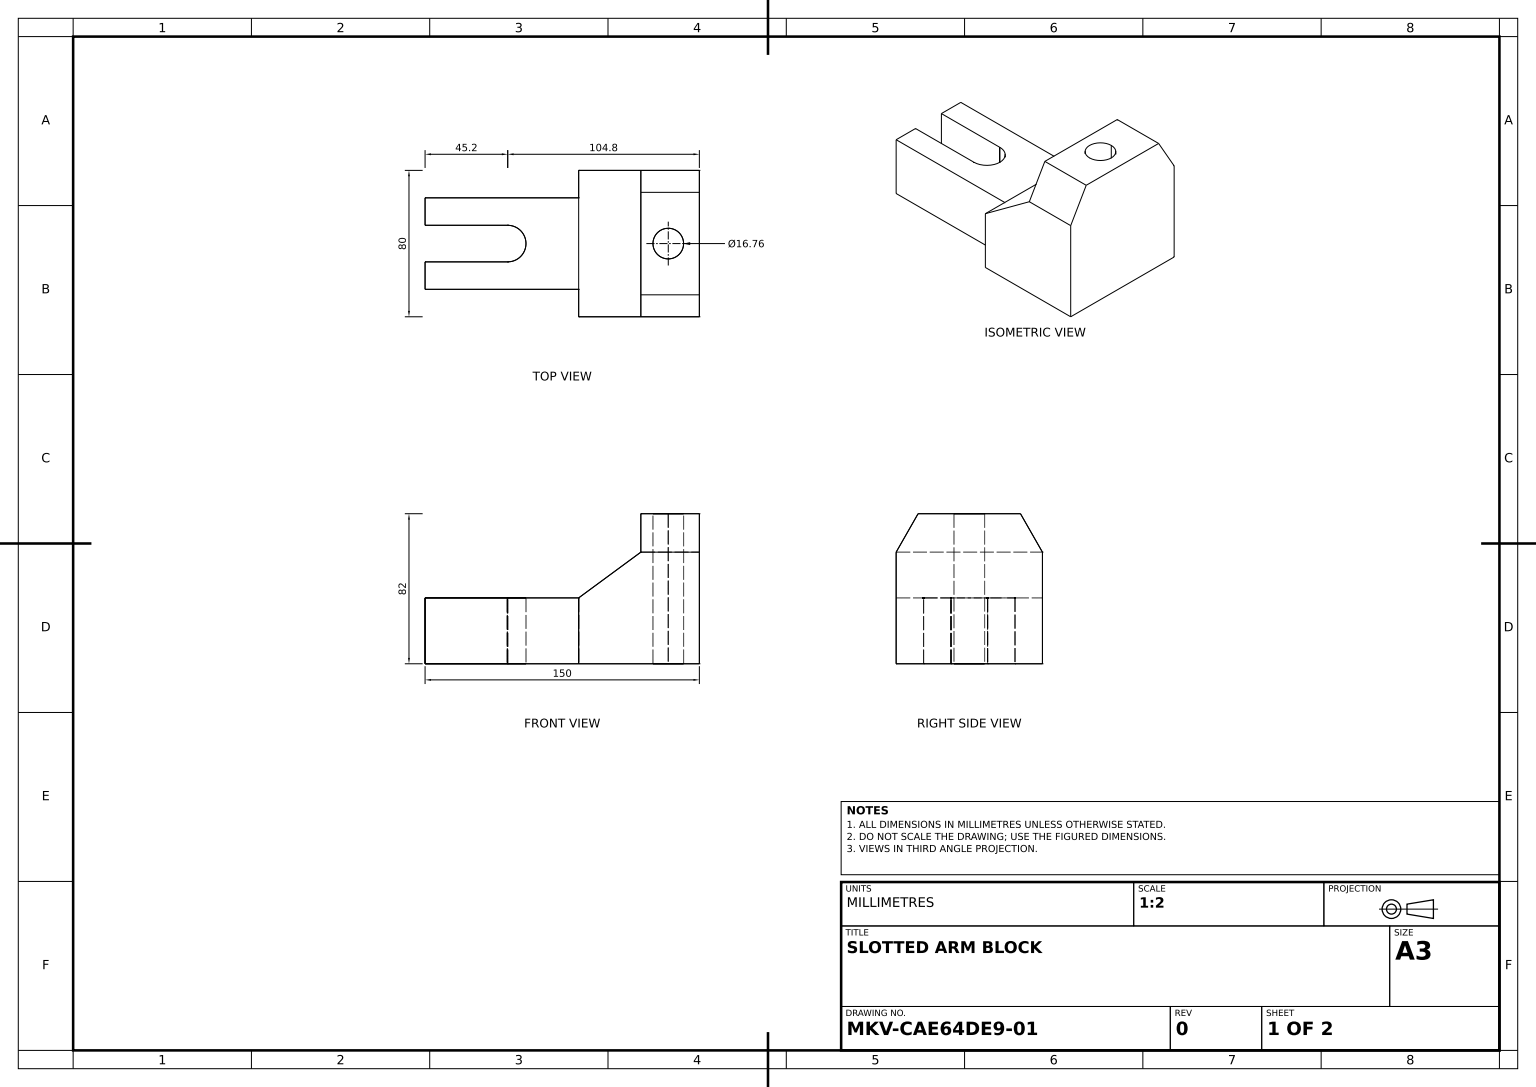
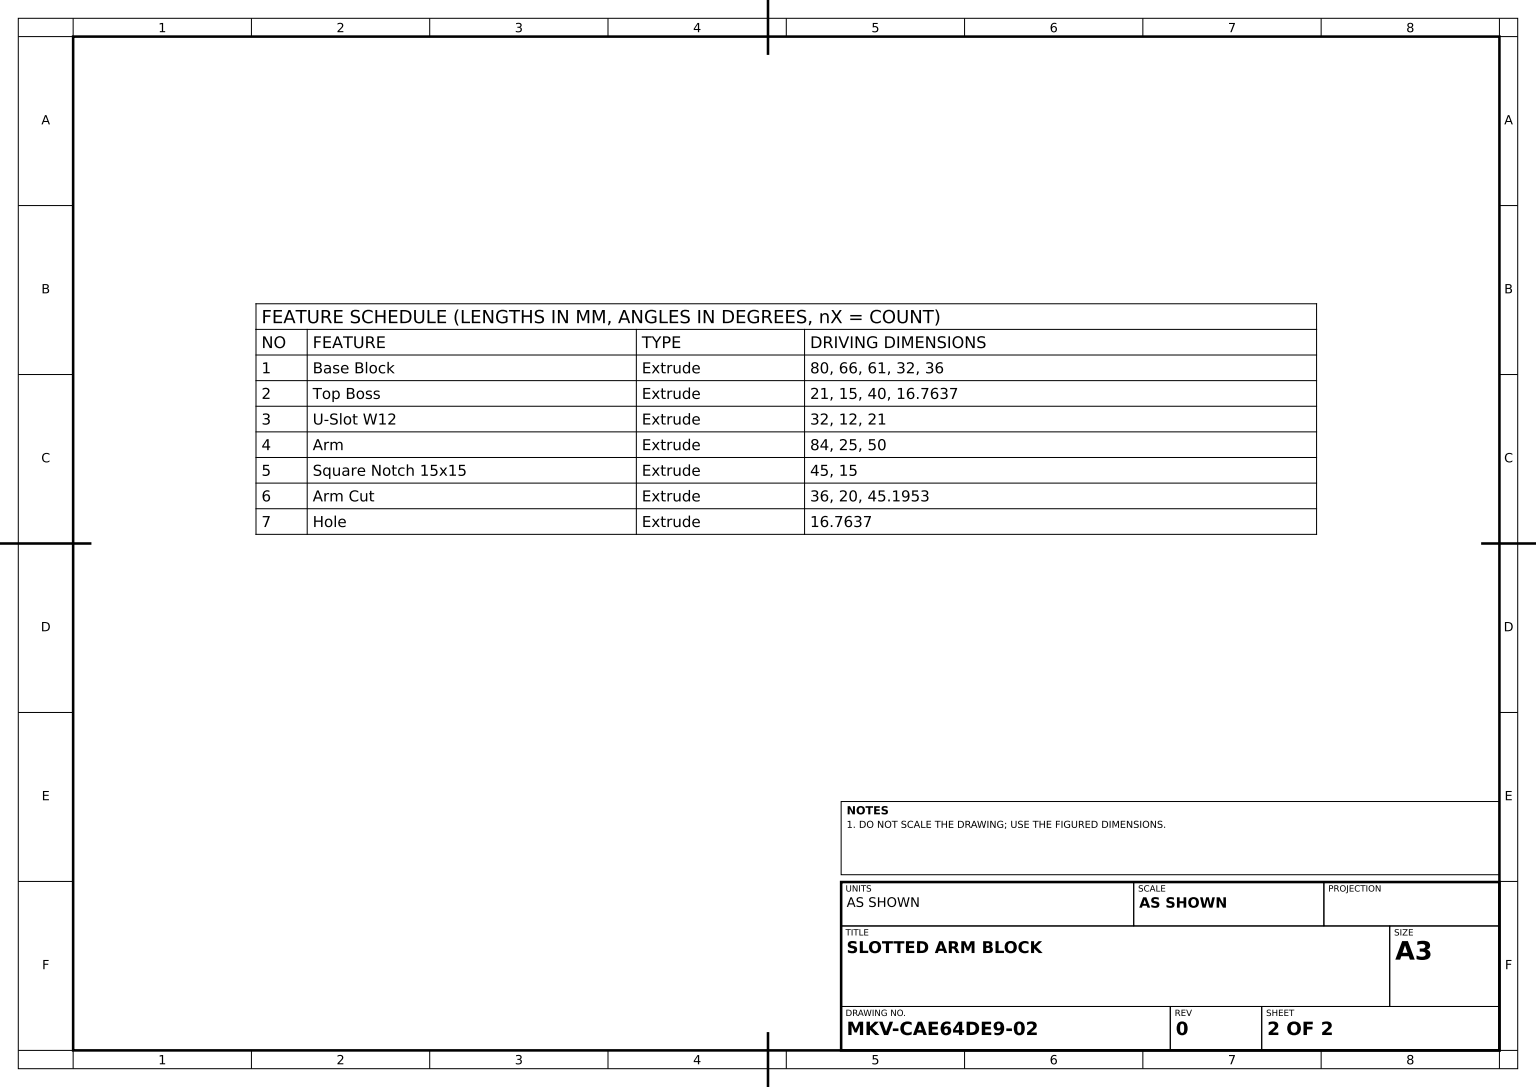
SolidWorks part; units mm, degrees
material "Plain Carbon Steel"
ref_plane "Front Plane" through (0, 0, 0) normal (0, 0, 1) x (1, 0, 0)
ref_plane "Top Plane" through (0, 0, 0) normal (0, 1, 0) x (1, 0, 0)
ref_plane "Right Plane" through (0, 0, 0) normal (1, 0, 0) x (0, 0, -1)
sketch "Base Block Profile" plane through (0, 0, 0) normal (0, 0, 1) x (1, 0, 0)
  line L0 (0, 0) -> (0, 36)
  line L1 (0, 36) -> (34, 61)
  line L2 (34, 61) -> (66, 61)
  line L3 (66, 61) -> (66, 0)
  line L4 (66, 0) -> (0, 0)
  dimension "D1" = 66
  dimension "D2" = 61
  dimension "D3" = 32
  dimension "D4" = 34
  dimension "D5" = 36
extrude "Base Block" add sketch "Base Block Profile" along normal mid plane 80
sketch "Top Boss Profile" plane through (0, 61, 0) normal (0, 1, 0) x (1, 0, 0)
  line L0 (34, 40) -> (66, 40)
  line L1 (66, 40) -> (66, -40)
  line L2 (66, -40) -> (34, -40)
  line L3 (34, -40) -> (34, 40)
  circle A0 centre (49, 0) radius 8.3819
  point P10 (34, 0)
  dimension "D1" = 15
  dimension "D3" = 16.7637
  dimension "D2" = 40
extrude "Top Boss" add sketch "Top Boss Profile" along normal blind 21
sketch "U-Slot Profile" plane through (66, 0, 0) normal (1, 0, 0) x (0, 0, -1)
  line L0 (0, 0) -> (0, 84.9134) construction
  line L1 (-40, 82) -> (-28, 82)
  line L2 (-40, 82) -> (40, 82) construction
  line L3 (40, 61) -> (28, 82)
  line L4 (-40, 82) -> (-40, 61)
  line L5 (-40, 0) -> (-40, 82) construction
  line L6 (-40, 61) -> (-28, 82)
  line L7 (40, 82) -> (40, 61)
  line L8 (40, 82) -> (28, 82)
  dimension "D1" = 12
  dimension "D2" = 21
extrude "U-Slot W12" cut sketch "U-Slot Profile" against normal blind 32
sketch "Arm Profile" plane through (0, 0, 0) normal (-1, 0, 0) x (0, 0, 1)
  line L0 (40, 36) -> (-40, 36) construction
  line L1 (-25, 36) -> (25, 36)
  line L2 (-25, 36) -> (-25, 0)
  line L3 (-25, 0) -> (25, 0)
  line L4 (25, 36) -> (25, 0)
  line L5 (40, 0) -> (-40, 0) construction
  dimension "D1" = 25
  dimension "D2" = 50
  dimension "D3" = 36
extrude "Arm" add sketch "Arm Profile" along normal blind 84
sketch "Square Notch Profile" plane through (-84, 0, 0) normal (-1, 0, 0) x (0, 0, 1)
  line L0 (25, 36) -> (-25, 36) construction
  line L1 (-10, 36) -> (10, 36)
  line L2 (-10, 36) -> (-10, 0)
  line L3 (-10, 0) -> (10, 0)
  line L4 (10, 36) -> (10, 0)
  line L5 (-25, 0) -> (25, 0) construction
  dimension "D1" = 15
  dimension "D2" = 15
extrude "Square Notch 15x15" cut sketch "Square Notch Profile" against normal blind 45
sketch "Arm Cut Profile" plane through (0, 36, 0) normal (0, 1, 0) x (1, 0, 0)
  line L0 (0, 0) -> (-73.7822, 0) construction
  line L1 (-84, 10) -> (-84, 25) construction
  circle A0 centre (-38.8047, 0) radius 10
  dimension "D1" = 20
  dimension "D2" = 45.1953
extrude "Arm Cut" cut sketch "Arm Cut Profile" against normal blind 36
sketch "Hole Sketch" plane through (0, 82, 0) normal (0, 1, 0) x (1, 0, 0)
  circle A0 centre (49, 0) radius 8.3819
  dimension "D1" = 16.7637
extrude "Hole" cut sketch "Hole Sketch" against normal through all
